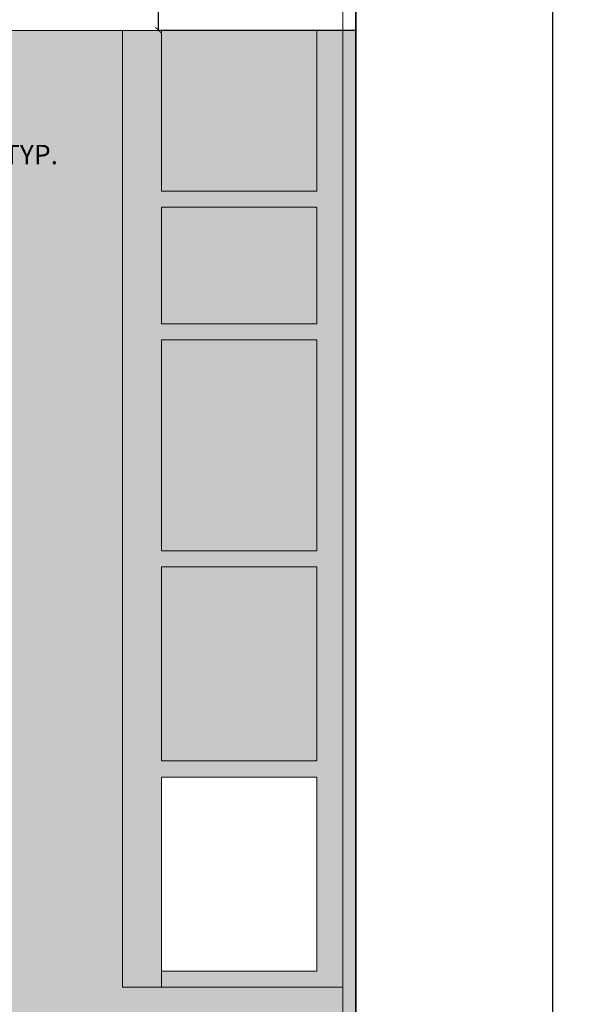
# Model space of a CAD drawing. Units: inches. Extents: x 1704 to 6393, y -157 to 1172.
# Tile 38 of 122: x 2619 to 2793, y 67 to 372. Entities that reach past the tile are written whole.
import ezdxf

# ---------------------------------------------------------------- set-up
doc = ezdxf.new("R2010")
doc.units = ezdxf.units.IN
doc.header["$MEASUREMENT"] = 0
for name, color, linetype, lineweight in [('A-ANNO-DIMS', 7, 'Continuous', 13), ('A-WALL-PATT', 7, 'Continuous', 13), ('C-PROP', 7, 'Continuous', 35), ('L-HRDS', 8, 'Continuous', 18), ('L-PVMT-PATT', 8, 'Continuous', 13)]:
    doc.layers.add(name, color=color, linetype=linetype, lineweight=lineweight)
doc.layers.add('L-HRDS-PATT', color=9, linetype='Continuous', lineweight=13, true_color=0xc5c1ba)
doc.styles.get("Standard").update_dxf_attribs({"font": 'arial.ttf'})
doc.dimstyles.get("Standard").update_dxf_attribs({"dimtxt": 6, "dimasz": 2, "dimexe": 0.18, "dimexo": 0.0625, "dimgap": 0.09, "dimtad": 0, "dimtih": 1, "dimtoh": 1, "dimdec": 1, "dimzin": 0, "dimdsep": 46, "dimlunit": 3, "dimtxsty": 'Standard', "dimblk": 'ARCHTICK', "dimcen": 0.09, "dimadec": 0, "dimazin": 0, "dimtfac": 1, "dimtdec": 1, "dimtofl": 0, "dimtmove": 0, "dimatfit": 3, "dimfxl": 1, "dimtolj": 1, "dimtzin": 0, "dimarcsym": 0})

# ---------------------------------------------------------------- blocks, each defined once
blk = doc.blocks.new('_ArchTick')
at = {"color": 0, "linetype": 'ByBlock', "const_width": 0.15}
blk.add_lwpolyline([(-0.5, -0.5), (0.5, 0.5)], dxfattribs=at)
blk = doc.blocks.new('*D43')
at = {"layer": 'A-ANNO-DIMS', "color": 0, "lineweight": -2, "transparency": 16777216}
for p, q in [((2597.35, 326.28), (2597.35, 329.99)), ((2597.35, 329.81), (2605.35, 329.81)), ((2605.35, 326.28), (2605.35, 329.99)), ((2605.35, 329.81), (2607.35, 329.81))]:
    blk.add_line(p, q, dxfattribs=at)
at = {"layer": 'Defpoints', "color": 0, "lineweight": -3, "transparency": 16777216}
for p in [(2605.35, 329.81), (2597.35, 326.21), (2605.35, 326.21)]:
    blk.add_point(p, dxfattribs=at)
at = {"layer": 'A-ANNO-DIMS', "color": 0, "lineweight": -2, "transparency": 16777216, "xscale": 2, "yscale": 2, "zscale": 2, "rotation": 180}
blk.add_blockref('_ArchTick', (2597.35, 329.81), dxfattribs=at)
at = {"layer": 'A-ANNO-DIMS', "color": 0, "lineweight": -2, "transparency": 16777216, "xscale": 2, "yscale": 2, "zscale": 2}
blk.add_blockref('_ArchTick', (2605.35, 329.81), dxfattribs=at)
at = {"layer": 'A-ANNO-DIMS', "color": 0, "transparency": 16777216, "insert": (2619.71, 329.81), "char_height": 6, "attachment_point": 5}
blk.add_mtext('\\A1;8 TYP.', dxfattribs=at)
blk = doc.blocks.new('*D91')
at = {"layer": 'A-ANNO-DIMS', "color": 0, "lineweight": -2, "transparency": 16777216}
for p, q in [((2723.41, 1033.21), (2784.53, 1033.21)), ((2784.35, 1033.21), (2784.35, 517.87)), ((2784.35, -3.79), (2784.35, 511.56)), ((2723.41, -3.79), (2784.53, -3.79))]:
    blk.add_line(p, q, dxfattribs=at)
at = {"layer": 'Defpoints', "color": 0, "lineweight": -3, "transparency": 16777216}
for p in [(2723.35, 1033.21), (2784.35, 1033.21), (2723.35, -3.79)]:
    blk.add_point(p, dxfattribs=at)
at = {"layer": 'A-ANNO-DIMS', "color": 0, "lineweight": -2, "transparency": 16777216, "xscale": 2, "yscale": 2, "zscale": 2}
for p, rotation in [((2784.35, 1033.21), 90), ((2784.35, -3.79), 270)]:
    blk.add_blockref('_ArchTick', p, dxfattribs=dict(at, rotation=rotation))
at = {"layer": 'A-ANNO-DIMS', "color": 0, "transparency": 16777216, "insert": (2784.35, 514.71), "char_height": 6, "attachment_point": 5}
blk.add_mtext('\\A1;1037', dxfattribs=at)
blk = doc.blocks.new('*D97')
at = {"layer": 'A-ANNO-DIMS', "color": 0, "lineweight": -2, "transparency": 16777216}
for p, q in [((2723.29, 716.21), (2662.17, 716.21)), ((2662.35, 716.21), (2662.35, 545.37)), ((2662.35, 368.21), (2662.35, 539.06)), ((2723.29, 368.21), (2662.17, 368.21))]:
    blk.add_line(p, q, dxfattribs=at)
at = {"layer": 'Defpoints', "color": 0, "lineweight": -3, "transparency": 16777216}
for p in [(2662.35, 716.21), (2723.35, 716.21), (2723.35, 368.21)]:
    blk.add_point(p, dxfattribs=at)
at = {"layer": 'A-ANNO-DIMS', "color": 0, "lineweight": -2, "transparency": 16777216, "xscale": 2, "yscale": 2, "zscale": 2}
for p, rotation in [((2662.35, 716.21), 90), ((2662.35, 368.21), 270)]:
    blk.add_blockref('_ArchTick', p, dxfattribs=dict(at, rotation=rotation))
at = {"layer": 'A-ANNO-DIMS', "color": 0, "transparency": 16777216, "insert": (2662.35, 542.21), "char_height": 6, "attachment_point": 5}
blk.add_mtext('\\A1;348', dxfattribs=at)

msp = doc.modelspace()

# ---------------------------------------------------------------- hatches: boundary and pattern name
at = {"layer": 'A-WALL-PATT', "transparency": 33554643}
h = msp.add_hatch(color=256, dxfattribs=at)
h.dxf.hatch_style = 1
h.paths.add_polyline_path([(2723.349, 368.213), (2719.349, 368.213), (2719.349, 5.658), (2719.349, -3.787), (2723.349, -3.787)])
at = {"layer": 'L-HRDS-PATT', "transparency": 33554539}
h = msp.add_hatch(color=256, dxfattribs=at)
h.dxf.hatch_style = 1
h.paths.add_polyline_path([(2651.217, 368.213), (2605.349, 368.213), (2605.349, 218.213), (2605.349, 212.464), (2605.349, 210.513), (2605.349, 153.913), (2605.349, 151.962), (2605.349, 146.213), (2605.349, 90.213), (2605.349, 72.213), (2601.349, 72.213), (2600.88, 50.634), (2719.349, 50.634), (2719.349, 72.213), (2711.349, 72.213), (2663.217, 72.213), (2651.217, 72.213)])
h.paths.add_polyline_path([(2711.349, 48.634), (2600.88, 48.634), (2576.88, 48.634), (2576.88, 17.658), (2711.349, 17.658)])
h.paths.add_polyline_path([(2601.349, 72.213), (2597.349, 72.213), (2597.349, 90.213), (2429.349, 90.213), (2425.516, 90.213), (2424.215, 90.213), (2386.482, 90.213), (2385.181, 90.213), (2381.349, 90.213), (2357.349, 90.213), (2357.349, 72.213), (2349.349, 72.213), (2349.349, 90.213), (2349.349, 134.213), (2277.349, 134.213), (2277.349, 50.634), (2566.88, 50.634), (2600.88, 50.634)])
h.paths.add_polyline_path([(2349.349, 146.213), (2277.349, 146.213), (2277.349, 134.213), (2349.349, 134.213)])
h.paths.add_polyline_path([(2349.349, 158.213), (2277.349, 158.213), (2277.349, 146.213), (2349.349, 146.213)])
h.paths.add_polyline_path([(2349.349, 170.213), (2277.349, 170.213), (2277.349, 158.213), (2349.349, 158.213)])
h.paths.add_polyline_path([(2349.349, 194.213), (2337.349, 194.213), (2337.349, 202.213), (2349.349, 202.213), (2349.349, 364.213), (2277.349, 364.213), (2277.349, 202.213), (2289.349, 202.213), (2289.349, 194.213), (2277.349, 194.213), (2277.349, 170.213), (2349.349, 170.213)])
at = {"layer": 'L-HRDS-PATT', "transparency": 33554528}
h = msp.add_hatch(color=256, dxfattribs=at)
h.dxf.hatch_style = 1
h.paths.add_polyline_path([(2711.349, 368.213), (2663.217, 368.213), (2663.217, 318.481), (2711.349, 318.481)])
h.paths.add_polyline_path([(2711.349, 313.481), (2663.217, 313.481), (2663.217, 277.481), (2711.349, 277.481)])
h.paths.add_polyline_path([(2711.349, 272.481), (2663.217, 272.481), (2663.217, 207.213), (2711.349, 207.213)])
h.paths.add_polyline_path([(2711.349, 202.213), (2663.217, 202.213), (2663.217, 142.213), (2711.349, 142.213)])
at = {"layer": 'L-PVMT-PATT', "transparency": 33554643}
h = msp.add_hatch(dxfattribs=at)
h.set_pattern_fill('GRAVEL', color=256, scale=2.4)
h.set_pattern_definition([(228.0127875, (1.728, 2.4), (-19.2, -21.6), [0.3228864, -31.9658113]), (184.9697407, (1.512, 2.16), (28.8, 2.4), [0.5540832, -54.8542194]), (132.510447, (0.96, 2.112), (24, -26.4), [0.3906912, -38.6784782]), (267.273689, (0.024, 1.512), (2.4, 48), [0.5045712, -49.9525393]), (292.833654, (0, 1.008), (-12, 28.8), [0.494772, -48.9824955]), (357.273689, (0.192, 0.552), (-48, 2.4), [0.5045712, -49.9525393]), (37.6942405, (0.696, 0.528), (-31.2, -24), [0.6672696, -66.0596365]), (72.2553284, (1.224, 0.936), (16.8, 52.8), [0.6299712, -62.3671716]), (121.4295656, (1.416, 1.536), (-19.2, 31.2), [0.50628, -50.1217755]), (175.236358, (1.152, 1.968), (26.4, -2.4), [0.5779968, -28.3218302]), (222.3974378, (0.576, 2.016), (-28.8, -26.4), [0.7474752, -74.0001]), (138.814075, (2.4, 1.488), (-16.8, 14.4), [0.2551224, -25.2572276]), (171.4692344, (2.208, 1.656), (31.2, -4.8), [0.4853688, -48.0516274]), (225, (1.728, 1.728), (-3e-16, -2.4), [0.3394104, -3.0547021]), (203.19859, (1.56, 2.016), (12, 4.8), [0.1827792, -18.0950763]), (291.80141, (1.392, 1.944), (-2.4, 7.2), [0.2584872, -12.6659083]), (30.963757, (1.488, 1.704), (7.2, 4.8), [0.4198296, -13.574455]), (161.56505, (1.848, 1.92), (4.8, -2.4), [0.3035784, -7.285888]), (16.3895403, (0, 1.944), (24, 7.2), [0.42528, -42.1028284]), (70.346176, (0.408, 2.064), (-9.6, -26.4), [0.3567864, -35.3217786]), (293.19859, (1.848, 2.4), (-4.8, 12), [0.365556, -17.9122995]), (343.6104597, (1.992, 2.064), (-24, 7.2), [0.42528, -42.1028284]), (339.443955, (0, 0.456), (-12, 4.8), [0.410112, -20.095497]), (294.7751406, (0.384, 0.312), (-12, 26.4), [0.3436272, -34.0191434]), (66.80141, (1.872, 0), (4.8, 12), [0.365556, -17.9122995]), (17.3540246, (2.016, 0.336), (-31.2, -9.6), [0.4023144, -39.8290167]), (69.443955, (0.696, 0), (-4.8, -12), [0.205056, -20.300553]), (101.309932, (1.728, 0), (-2.4, 9.6), [0.122376, -12.1152708]), (165.963757, (1.704, 0.12), (7.2, -2.4), [0.494772, -9.4006815]), (186.009006, (1.224, 0.24), (24, 2.4), [0.45852, -45.3934156]), (303.690068, (1.488, 1.488), (-2.4, 4.8), [0.3461328, -8.3071903]), (353.1572266, (1.68, 1.2), (40.8, -4.8), [0.6043056, -59.8261503]), (60.945396, (2.28, 1.128), (-9.6, -16.8), [0.2470944, -24.462418]), (90, (2.4, 1.344), (-2.4, 2.4), [0.144, -2.256]), (120.256437, (1.176, 0.312), (9.6, -16.8), [0.3334176, -33.008448]), (48.0127875, (1.008, 0.6), (19.2, 21.6), [0.6457728, -31.642925]), (0, (1.44, 1.08), (2.4, 2.4), [0.624, -1.776]), (325.3048465, (2.064, 1.08), (24, -16.8), [0.3794736, -37.5678583]), (254.054604, (2.376, 0.864), (-2.4, -9.6), [0.3494448, -17.122819]), (207.6459754, (2.28, 0.528), (-45.6, -24), [0.568956, -56.326738]), (175.4260787, (1.776, 0.264), (-31.2, 2.4), [0.6019176, -59.5897762])])
h.paths.add_polyline_path([(2719.349, 368.213), (2711.349, 368.213), (2711.349, 318.481), (2663.217, 318.481), (2663.217, 368.213), (2651.217, 368.213), (2651.217, 72.213), (2663.217, 72.213), (2663.217, 137.213), (2711.349, 137.213), (2711.349, 72.213), (2663.217, 72.213), (2651.217, 72.213), (2651.217, 368.213), (2605.349, 368.213), (2605.349, 218.213), (2605.349, 212.464), (2605.349, 210.513), (2605.349, 153.913), (2605.349, 151.962), (2605.349, 146.213), (2605.349, 90.213), (2605.349, 72.213), (2601.349, 72.213), (2600.88, 50.634), (2277.349, 50.634), (2277.349, -3.787), (2719.349, -3.787)])
h.paths.add_polyline_path([(2663.217, 272.481), (2711.349, 272.481), (2711.349, 207.213), (2663.217, 207.213)], flags=16)
h.paths.add_polyline_path([(2663.217, 202.213), (2711.349, 202.213), (2711.349, 142.213), (2663.217, 142.213)], flags=16)
h.paths.add_polyline_path([(2663.217, 277.481), (2663.217, 313.481), (2711.349, 313.481), (2711.349, 277.481)], flags=16)
h = msp.add_hatch(dxfattribs=at)
h.set_pattern_fill('GRAVEL', color=256, scale=10)
h.set_pattern_definition([(228.012788, (7.2, 10), (-80, -90), [1.34536, -133.19088]), (184.96974, (6.3, 9), (120, 10), [2.30868, -228.559248]), (132.510447, (4, 8.8), (100, -110), [1.62788, -161.160326]), (267.273689, (0.1, 6.3), (10, 200), [2.10238, -208.13558]), (292.833654, (0, 4.2), (-50, 120), [2.06155, -204.09373]), (357.273689, (0.8, 2.3), (-200, 10), [2.10238, -208.13558]), (37.69424, (2.9, 2.2), (-130, -100), [2.78029, -275.248485]), (72.255328, (5.1, 3.9), (70, 220), [2.62488, -259.863215]), (121.429566, (5.9, 6.4), (-80, 130), [2.1095, -208.84073]), (175.23636, (4.8, 8.2), (110, -10), [2.40832, -118.007626]), (222.397438, (2.4, 8.4), (-120, -110), [3.11448, -308.33375]), (138.814075, (10, 6.2), (-70, 60), [1.06301, -105.238448]), (171.469234, (9.2, 6.9), (130, -20), [2.02237, -200.215114]), (225, (7.2, 7.2), (-1e-15, -10), [1.41421, -12.727926]), (203.19859, (6.5, 8.4), (50, 20), [0.76158, -75.39615]), (291.80141, (5.8, 8.1), (-10, 30), [1.07703, -52.774618]), (30.96376, (6.2, 7.1), (30, 20), [1.74929, -56.56023]), (161.56505, (7.7, 8), (20, -10), [1.26491, -30.357867]), (16.38954, (0, 8.1), (100, 30), [1.772, -175.42845]), (70.346176, (1.7, 8.6), (-40, -110), [1.48661, -147.174077]), (293.19859, (7.7, 10), (-20, 50), [1.52315, -74.63458]), (343.61046, (8.3, 8.6), (-100, 30), [1.772, -175.42845]), (339.443955, (0, 1.9), (-50, 20), [1.7088, -83.731237]), (294.77514, (1.6, 1.3), (-50, 110), [1.43178, -141.74643]), (66.80141, (7.8, 0), (20, 50), [1.52315, -74.63458]), (17.354025, (8.4, 1.4), (-130, -40), [1.67631, -165.954236]), (69.443955, (2.9, 0), (-20, -50), [0.8544, -84.585637]), (101.30993, (7.2, 0), (-10, 40), [0.5099, -50.480295]), (165.96376, (7.1, 0.5), (30, -10), [2.06155, -39.169506]), (186.009006, (5.1, 1), (100, 10), [1.9105, -189.139232]), (303.69007, (6.2, 6.2), (-10, 20), [1.44222, -34.613293]), (353.157227, (7, 5), (170, -20), [2.51794, -249.275626]), (60.945396, (9.5, 4.7), (-40, -70), [1.02956, -101.92674]), (90, (10, 5.6), (-10, 10), [0.6, -9.4]), (120.256437, (4.9, 1.3), (40, -70), [1.38924, -137.5352]), (48.012788, (4.2, 2.5), (80, 90), [2.69072, -131.84552]), (0, (6, 4.5), (10, 10), [2.6, -7.4]), (325.304846, (8.6, 4.5), (100, -70), [1.58114, -156.532743]), (254.054604, (9.9, 3.6), (-10, -40), [1.45602, -71.34508]), (207.645975, (9.5, 2.2), (-190, -100), [2.37065, -234.694742]), (175.426079, (7.4, 1.1), (-130, 10), [2.50799, -248.290734])])
h.paths.add_polyline_path([(2719.349, 368.213), (2711.349, 368.213), (2711.349, 318.481), (2663.217, 318.481), (2663.217, 368.213), (2651.217, 368.213), (2651.217, 72.213), (2663.217, 72.213), (2663.217, 137.213), (2711.349, 137.213), (2711.349, 77.213), (2663.217, 77.213), (2663.217, 72.213), (2711.349, 72.213), (2719.349, 72.213)])
h.paths.add_polyline_path([(2663.217, 202.213), (2711.349, 202.213), (2711.349, 142.213), (2663.217, 142.213)], flags=16)
h.paths.add_polyline_path([(2663.217, 207.213), (2663.217, 272.481), (2711.349, 272.481), (2711.349, 207.213)], flags=16)
h.paths.add_polyline_path([(2663.217, 277.481), (2663.217, 313.481), (2711.349, 313.481), (2711.349, 277.481)], flags=16)

# ---------------------------------------------------------------- linework, layer by layer
at = {"layer": 'C-PROP'}
msp.add_line((2723.349, -3.787), (2723.349, 1033.213), dxfattribs=at)
at = {"layer": 'L-HRDS'}
for p, q in [((2719.349, 5.658), (2719.349, 1033.213)), ((2605.349, 368.213), (2651.217, 368.213)), ((2651.217, 368.213), (2651.217, 72.213)), ((2651.217, 368.213), (2663.217, 368.213)), ((2663.217, 368.213), (2663.217, 318.481)), ((2663.217, 368.213), (2723.349, 368.213)), ((2711.349, 318.481), (2711.349, 368.213)), ((2663.217, 318.481), (2711.349, 318.481)), ((2663.217, 313.481), (2711.349, 313.481)), ((2663.217, 313.481), (2663.217, 277.481)), ((2711.349, 277.481), (2711.349, 313.481)), ((2663.217, 277.481), (2711.349, 277.481)), ((2663.217, 272.481), (2711.349, 272.481)), ((2663.217, 272.481), (2663.217, 207.213)), ((2711.349, 207.213), (2711.349, 272.481)), ((2663.217, 207.213), (2711.349, 207.213)), ((2663.217, 202.213), (2711.349, 202.213)), ((2663.217, 202.213), (2663.217, 142.213)), ((2711.349, 142.213), (2711.349, 202.213)), ((2663.217, 142.213), (2711.349, 142.213)), ((2663.217, 137.213), (2711.349, 137.213)), ((2663.217, 137.213), (2663.217, 72.213)), ((2711.349, 77.213), (2711.349, 137.213)), ((2663.217, 77.213), (2711.349, 77.213)), ((2651.217, 72.213), (2663.217, 72.213)), ((2663.217, 72.213), (2711.349, 72.213)), ((2711.349, 72.213), (2719.349, 72.213))]:
    msp.add_line(p, q, dxfattribs=at)

# ---------------------------------------------------------------- dimensions: what is measured, and where the dimension line sits
at = {"layer": 'A-ANNO-DIMS'}
for base, p1, p2, picture, middle in [((2784.349, 1033.213), (2723.349, -3.787), (2723.349, 1033.213), '*D91', (2784.349, 514.713)), ((2662.349, 716.213), (2723.349, 368.213), (2723.349, 716.213), '*D97', (2662.349, 542.213))]:
    dim = msp.add_linear_dim(base=base, p1=p1, p2=p2, angle=90, dimstyle='Standard', override={"dimdec": 0, "dimlfac": 1, "dimrnd": 0, "dimzin": 0, "dimdsep": 46, "dimlunit": 2}, dxfattribs=at)
    dim.commit()
    dim.dimension.update_dxf_attribs({"geometry": picture, "text_midpoint": middle})
dim = msp.add_linear_dim(base=(2605.349, 329.813), p1=(2597.349, 326.213), p2=(2605.349, 326.213), text='<> TYP.', dimstyle='Standard', override={"dimdec": 0, "dimlfac": 1, "dimrnd": 0, "dimzin": 0, "dimdsep": 46, "dimlunit": 2}, dxfattribs=at)
dim.commit()
dim.dimension.update_dxf_attribs({"geometry": '*D43', "text_midpoint": (2619.715, 329.813)})

doc.saveas('drawing.dxf')
